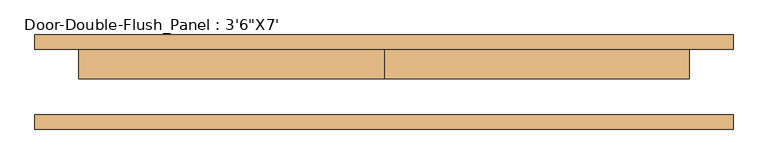
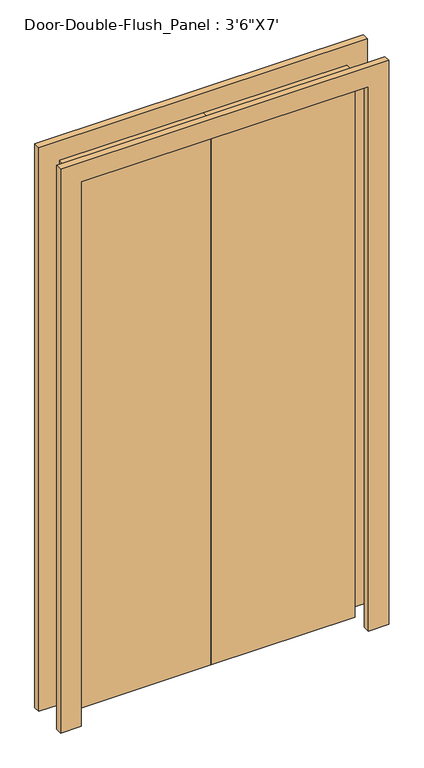
"""IFC4 building model written with IfcOpenShell, lengths in millimetres: door geometry."""

from ifc_helpers import new_model, si_unit, frame, origin, origin_with_axes, place, context, project, spatial, polyline, outline, extrude, source, transform, mapped, element, save


def door_d57fbbae(model_context):
    return source(origin(), model_context, "Body", "SweptSolid", [
        extrude(outline(polyline([(2133.6, -533.4), (2133.6, 533.4), (0.0, 533.4), (0.0, 609.6), (2209.8, 609.6), (2209.8, -609.6), (0.0, -609.6), (0.0, -533.4), (2133.6, -533.4)])), frame((0.0, 57.15, 0.0), z_axis=(0.0, 1.0, 0.0), x_axis=(0.0, 0.0, 1.0)), (0.0, 0.0, 1.0), 25.4),
        extrude(outline(polyline([(2133.6, -533.4), (2133.6, 533.4), (0.0, 533.4), (0.0, 609.6), (2209.8, 609.6), (2209.8, -609.6), (0.0, -609.6), (0.0, -533.4), (2133.6, -533.4)])), frame((0.0, -82.55, 0.0), z_axis=(0.0, 1.0, 0.0), x_axis=(0.0, 0.0, 1.0)), (0.0, 0.0, 1.0), 25.4),
        extrude(outline(polyline([(-533.4, 57.15), (0.0, 57.15), (0.0, 6.35), (-533.4, 6.35), (-533.4, 57.15)])), origin_with_axes(), (0.0, 0.0, 1.0), 2133.6),
        extrude(outline(polyline([(0.0, 57.15), (533.4, 57.15), (533.4, 6.35), (0.0, 6.35), (0.0, 57.15)])), origin_with_axes(), (0.0, 0.0, 1.0), 2133.6),
    ])


if __name__ == "__main__":
    model = new_model("IFC4")
    model_context = context("Model", 3, world=origin())
    ifc_project = project(units=[si_unit("LENGTHUNIT", "METRE", prefix="MILLI")], contexts=[model_context])
    site = spatial("IfcSite", under=ifc_project)
    building = spatial("IfcBuilding", under=site)
    placement = place(None, origin())
    door_shape = door_d57fbbae(model_context)
    element("IfcDoor", 1, ObjectType="Door-Double-Flush_Panel : 3'6\"X7'", at=placement, inside=building, context=model_context, shape_type="MappedRepresentation", body=[
        mapped(door_shape, transform((0.0, 0.0, 0.0), x_axis=(1.0, 0.0, 0.0), y_axis=(0.0, 1.0, 0.0), z_axis=(0.0, 0.0, 1.0))),
    ])
    save(model, "model.ifc")

# Revit data of these elements
# Type "Door-Double-Flush_Panel : 3'6\"X7'"
#   Type Mark = "12"
#   Construction Type Id = "DOOR"
#   Assembly Code = "C1020"
#   Analytic Construction = "Wooden"
#   Thickness = 0' - 2"
#   Thermal Resistance (R) = 2.5876 (h·ft²·°F)/BTU
#   Swing Angle [instance default] = 90.00°
#   Panel Width = 1' - 9"
#   Heat Transfer Coefficient (U) = 0.3865 BTU/(h·ft²·°F)
#   Height = 7' - 0"
#   Trim Projection Ext = 0' - 1"
#   Trim Projection Int = 0' - 1"
#   Trim Width = 0' - 3"
#   Width = 3' - 6"
#   Define Thermal Properties by = 1
#   Panel Material = Wood - Birch - Solid Stained Light Low Gloss
#   Trim Material = Paint - Sienna
#   Visual Light Transmittance = 0
#   Solar Heat Gain Coefficient = 0
#   Function = (empty or 0)
#   Wall Closure = (empty or 0)
# Element 1 (IfcDoor, "Door-Double-Flush_Panel : 3'6\"X7'")
#   Materials on its faces: "Paint - Sienna", "Wood - Birch - Solid Stained Light Low Gloss"
# Materials
#   "Wood - Birch - Solid Stained Light Low Gloss": class "Wood", colour RGB 210 159 95, transparency 0, Cost = 0
#   "Paint - Sienna": colour RGB 118 70 51, transparency 0, Cost = 0
